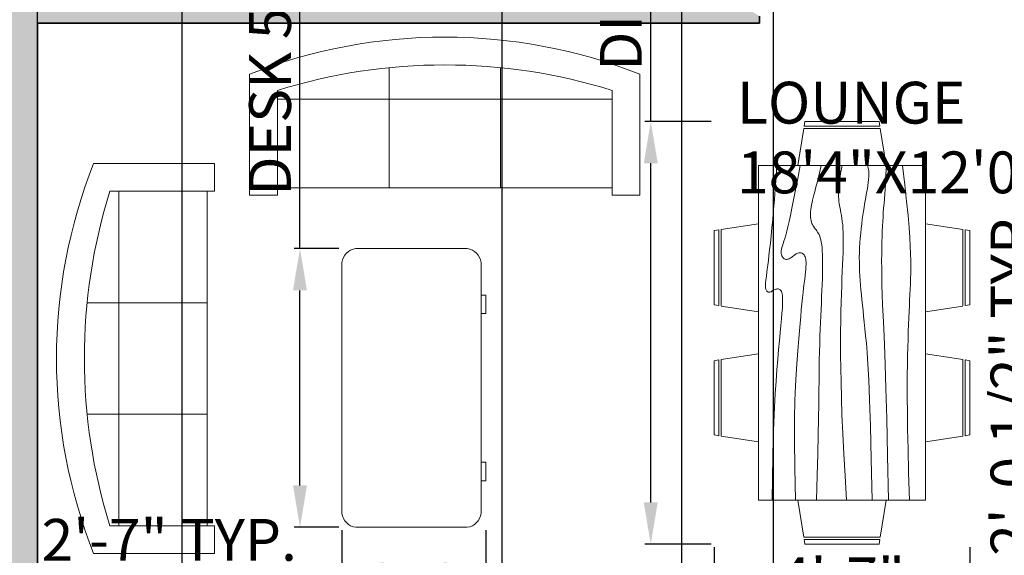
# Model space of a CAD drawing. Units: inches. Extents: x 32476 to 33108, y 58720 to 59630.
# Tile 4 of 6: x 32598 to 32810, y 59163 to 59278. Entities that reach past the tile are written whole.
import ezdxf

# ---------------------------------------------------------------- set-up
doc = ezdxf.new("R2010")
doc.units = ezdxf.units.IN
for name, color, linetype, lineweight in [('A-ANNO-DIMS', 6, 'Continuous', 18), ('A-AREA-IDEN', 32, 'Continuous', 18), ('A-FURN', 8, 'Continuous', 18), ('A-WALL', 7, 'Continuous', 35), ('A-WALL-PATT', 251, 'Continuous', 13)]:
    doc.layers.add(name, color=color, linetype=linetype, lineweight=lineweight)
doc.styles.get("Standard").update_dxf_attribs({"font": 'arial.ttf'})
doc.dimstyles.new('ISO-25', dxfattribs={"dimtxt": 9, "dimasz": 9, "dimexe": 1.25, "dimexo": 0.625, "dimtad": 1, "dimdec": 1, "dimrnd": 9, "dimlunit": 3, "dimtxsty": 'Standard', "dimcen": 2.5, "dimadec": 0, "dimazin": 0, "dimtfac": 1, "dimtdec": 1, "dimtmove": 0, "dimatfit": 3, "dimfxl": 1, "dimarcsym": 0})

# ---------------------------------------------------------------- blocks, each defined once
blk = doc.blocks.new('Sofa - Roundback 7 ft.')
for p, q in [((-12.00002, -32.4421), (-12.00003, -6.5971)), ((11.99997, -32.4421), (11.99998, -6.5971)), ((-36.000027, -34), (-36.000027, -11.4696)), ((35.99998, -34), (35.99998, -11.4696)), ((-35.999844, -13.3819), (35.9998, -13.3819)), ((-36.000027, -32.4421), (35.99998, -32.4421))]:
    blk.add_line(p, q)
for points in [[(-36.000027, -34), (-42.000027, -34), (-42.000027, -8)], [(41.99998, -8), (41.99998, -34), (35.99998, -34)]]:
    blk.add_lwpolyline(points)
for centre, radius, start, end in [((0, -114.25), 114.25, 68.43141, 111.5686), ((-0.00001, -127.1968), 121.1968, 72.72033, 107.2797)]:
    blk.add_arc(centre, radius, start, end)
blk = doc.blocks.new('Desk - 30 x 60 in.')
for p, q in [((-26.999995, 0), (26.999995, 0)), ((-29.999995, -27), (-29.999995, -3)), ((29.999995, -3), (29.999995, -27)), ((26.999995, -30), (-26.999995, -30)), ((-20.000005, -30), (-20.000005, -31)), ((-20.000005, -31), (-16.000005, -31)), ((-16.000005, -31), (-16.000005, -30)), ((15.999995, -31), (15.999995, -30)), ((19.999995, -31), (15.999995, -31)), ((19.999995, -30), (19.999995, -31))]:
    blk.add_line(p, q)
for centre, start, end in [((-26.499995, -3.5), 98.1301, 171.8699), ((26.499995, -3.5), 8.130102, 81.8699), ((-26.499995, -26.5), 188.1301, 261.8699), ((26.499995, -26.5), 278.1301, 351.8699)]:
    blk.add_arc(centre, 3.535534, start, end)
blk = doc.blocks.new('Dining Set - 36 x 72 in.')
for p, q in [((-22.2343, 26.00059), (-23.4847, 17.99762)), ((-22.2304, 26), (-5.7608, 26)), ((-22, 27.5), (-22.1562, 26.50042)), ((-5.8416, 26.5), (-22.1534, 26.5)), ((-22, 27.5), (-6, 27.5)), ((-5.8437, 26.49966), (-6, 27.5)), ((-4.5152, 17.99762), (-5.7655, 25.99926)), ((5.7657, 26.00059), (4.5153, 17.99762)), ((5.7696, 26), (22.2392, 26)), ((6, 27.5), (5.8438, 26.50042)), ((22.1584, 26.5), (5.8466, 26.5)), ((6, 27.5), (22, 27.5)), ((22.1563, 26.49966), (22, 27.5)), ((23.4848, 17.99762), (22.2345, 25.99926)), ((36, 18), (-36, 18)), ((-36, 18), (-36, -18)), ((36, -18), (36, 18)), ((-44.0006, 8.23428), (-35.9976, 9.48474)), ((44.0006, 8.23428), (35.9976, 9.48474)), ((-45.5, 8), (-44.5004, 8.15617)), ((-45.5, 8), (-45.5, -8)), ((-44.5, -8.15843), (-44.5, 8.15338)), ((-44, 8.23041), (-44, -8.23915)), ((44, 8.23041), (44, -8.23915)), ((44.5, -8.15843), (44.5, 8.15338)), ((45.5, 8), (44.5005, 8.15617)), ((45.5, 8), (45.5, -8)), ((-44.4997, -8.15631), (-45.5, -8)), ((-35.9976, -9.48476), (-43.9993, -8.2345)), ((35.9976, -9.48476), (43.9993, -8.2345)), ((44.4997, -8.15631), (45.5, -8)), ((-36, -18), (36, -18)), ((-22.2343, -26.0006), (-23.4847, -17.99762)), ((-4.5152, -17.99762), (-5.7655, -25.99928)), ((5.7657, -26.0006), (4.5153, -17.99762)), ((23.4848, -17.99762), (22.2345, -25.99928)), ((-22.2304, -26), (-5.7608, -26)), ((-22, -27.5), (-22.1562, -26.50044)), ((-5.8416, -26.5), (-22.1534, -26.5)), ((-22, -27.5), (-6, -27.5)), ((-5.8437, -26.49967), (-6, -27.5)), ((5.7696, -26), (22.2392, -26)), ((6, -27.5), (5.8438, -26.50044)), ((22.1584, -26.5), (5.8466, -26.5)), ((6, -27.5), (22, -27.5)), ((22.1563, -26.49967), (22, -27.5))]:
    blk.add_line(p, q)
for points in [[(-36, 15), (-31.1772, 14.97754), (-26.8079, 14.91406), (-22.8538, 14.81543), (-19.276, 14.6875), (-16.0362, 14.53613), (-13.0957, 14.36718), (-10.4159, 14.18652), (-7.9583, 14), (-5.6904, 13.81315), (-3.6035, 13.63021), (-1.6954, 13.45508), (0.0365, 13.29166), (1.5945, 13.14388), (2.9811, 13.01562), (4.1988, 12.9108), (5.25, 12.83333), (6.1393, 12.78613), (6.8802, 12.76823), (7.4883, 12.77767), (7.9792, 12.8125), (8.3685, 12.87077), (8.6719, 12.95052), (8.9049, 13.0498), (9.0833, 13.16666), (9.2205, 13.29899), (9.3216, 13.44401), (9.3895, 13.59879), (9.4271, 13.76041), (9.4373, 13.92594), (9.4232, 14.09245), (9.3875, 14.257), (9.3333, 14.41666), (9.2638, 14.56917), (9.1836, 14.71484), (9.0975, 14.85465), (9.0104, 14.98958), (8.9272, 15.1206), (8.8529, 15.2487), (8.7922, 15.37483), (8.75, 15.5), (8.7305, 15.62467), (8.7344, 15.74739), (8.7617, 15.86621), (8.8125, 15.97916), (8.8867, 16.08431), (8.9844, 16.17968), (9.1055, 16.26334), (9.25, 16.33333), (9.4189, 16.38802), (9.6172, 16.42708), (9.8506, 16.45052), (10.125, 16.45833), (10.4463, 16.45052), (10.8203, 16.42708), (11.2529, 16.38802), (11.75, 16.33333), (12.3184, 16.26318), (12.9694, 16.17838), (13.7151, 16.07991), (14.5677, 15.96875), (15.5395, 15.84586), (16.6426, 15.71224), (17.8893, 15.56884), (19.2917, 15.41666), (20.859, 15.25667), (22.5879, 15.08984), (24.4721, 14.91715), (26.5052, 14.73958), (28.6809, 14.5581), (30.9929, 14.3737), (33.4347, 14.18733), (36, 14)], [(-36, 10), (-28.9766, 10.14274), (-23.1725, 10.20442), (-18.4241, 10.19775), (-14.5677, 10.13541), (-11.4399, 10.03011), (-8.877, 9.89453), (-6.7154, 9.74137), (-4.7917, 9.58333), (-2.9698, 9.43082), (-1.2246, 9.28515), (0.4415, 9.14534), (2.026, 9.01041), (3.5266, 8.87939), (4.9408, 8.7513), (6.266, 8.62516), (7.5, 8.5), (8.6411, 8.37549), (9.6914, 8.2539), (10.6538, 8.13818), (11.5312, 8.03125), (12.3267, 7.93603), (13.043, 7.85547), (13.6831, 7.79248), (14.25, 7.75), (14.7471, 7.7303), (15.1797, 7.73307), (15.5537, 7.75732), (15.875, 7.80208), (16.1494, 7.86637), (16.3828, 7.94922), (16.5811, 8.04964), (16.75, 8.16666), (16.8944, 8.29915), (17.0143, 8.44531), (17.1089, 8.60319), (17.1771, 8.77083), (17.218, 8.94629), (17.2305, 9.1276), (17.2137, 9.31282), (17.1667, 9.5), (17.0895, 9.6875), (16.987, 9.875), (16.8649, 10.0625), (16.7292, 10.25), (16.5856, 10.4375), (16.4401, 10.625), (16.2985, 10.8125), (16.1667, 11), (16.05, 11.18733), (15.9518, 11.3737), (15.8752, 11.5581), (15.8229, 11.73958), (15.798, 11.91715), (15.8034, 12.08984), (15.842, 12.25667), (15.9167, 12.41666), (16.0295, 12.56836), (16.1784, 12.70833), (16.3605, 12.83268), (16.5729, 12.9375), (16.8127, 13.01888), (17.0768, 13.07291), (17.3625, 13.0957), (17.6667, 13.08333), (17.9894, 13.03312), (18.3418, 12.94726), (18.7382, 12.82918), (19.1927, 12.68229), (19.7195, 12.51001), (20.3327, 12.31575), (21.0465, 12.10294), (21.875, 11.875), (22.8357, 11.63354), (23.959, 11.37304), (25.2786, 11.08618), (26.8282, 10.76562), (28.6414, 10.40405), (30.752, 9.99414), (33.1936, 9.52856), (36, 9)], [(-36, 5.5), (-30.7157, 5.3348), (-26.069, 5.20963), (-21.9946, 5.11767), (-18.4271, 5.05208), (-15.3009, 5.00602), (-12.5508, 4.97265), (-10.1112, 4.94515), (-7.9167, 4.91666), (-5.909, 4.88167), (-4.0586, 4.83984), (-2.3429, 4.79215), (-0.7396, 4.73958), (0.7739, 4.6831), (2.22, 4.6237), (3.6213, 4.56233), (5, 4.5), (6.373, 4.43782), (7.7344, 4.3776), (9.0723, 4.32129), (10.375, 4.27083), (11.6309, 4.22819), (12.8281, 4.19531), (13.9551, 4.17415), (15, 4.16666), (15.954, 4.17448), (16.819, 4.19791), (17.6001, 4.23698), (18.3021, 4.29166), (18.9299, 4.36198), (19.4883, 4.44791), (19.9823, 4.54948), (20.4167, 4.66666), (20.7969, 4.79899), (21.1302, 4.94401), (21.4245, 5.09879), (21.6875, 5.26041), (21.9271, 5.42594), (22.1511, 5.59245), (22.3672, 5.757), (22.5834, 5.91666), (22.8065, 6.06868), (23.0404, 6.21093), (23.2879, 6.34147), (23.5521, 6.45833), (23.8358, 6.55957), (24.142, 6.64323), (24.4735, 6.70735), (24.8334, 6.75), (25.2235, 6.76969), (25.642, 6.76692), (26.0858, 6.74267), (26.5521, 6.69791), (27.0379, 6.63362), (27.5404, 6.55078), (28.0565, 6.45036), (28.5834, 6.33333), (29.1242, 6.19987), (29.7071, 6.04687), (30.3661, 5.87044), (31.1354, 5.66666), (32.0493, 5.43164), (33.142, 5.16146), (34.4475, 4.85221), (36, 4.5)], [(-36, -1), (-30.7915, -0.6591), (-26.0195, -0.38216), (-21.6519, -0.16284), (-17.6563, 0.00521), (-14.0005, 0.12833), (-10.6523, 0.21289), (-7.5796, 0.26522), (-4.75, 0.29166), (-2.134, 0.29793), (0.2878, 0.28711), (2.5317, 0.26163), (4.6146, 0.22396), (6.5529, 0.17651), (8.3633, 0.12174), (10.0623, 0.06209), (11.6667, 0), (13.1899, -0.06201), (14.6341, -0.1211), (15.9982, -0.17432), (17.2813, -0.21875), (18.4823, -0.25147), (19.6003, -0.26953), (20.6343, -0.27002), (21.5834, -0.25), (22.4481, -0.20768), (23.2357, -0.14584), (23.9549, -0.06836), (24.6146, 0.02083), (25.2235, 0.11784), (25.7904, 0.21875), (26.3241, 0.31966), (26.8334, 0.41666), (27.3265, 0.50618), (27.8099, 0.58593), (28.2894, 0.65397), (28.7709, 0.70833), (29.2601, 0.74707), (29.763, 0.76823), (30.2855, 0.76985), (30.8334, 0.75), (31.4088, 0.70784), (31.9994, 0.64713), (32.589, 0.57275), (33.1615, 0.48958), (33.7008, 0.4025), (34.1908, 0.3164), (34.6153, 0.23616), (34.9584, 0.16666), (35.2099, 0.11165), (35.3848, 0.07031), (35.504, 0.04069), (35.5886, 0.02083), (35.6594, 0.00879), (35.7377, 0.0026), (35.8442, 0.00032), (36, 0)], [(-36, -6.5), (-27.1843, -6.31267), (-20.084, -6.1263), (-14.469, -5.9419), (-10.1094, -5.76042), (-6.7752, -5.58285), (-4.2363, -5.41016), (-2.2629, -5.24333), (-0.625, -5.08334), (0.8708, -4.93099), (2.2715, -4.78646), (3.5872, -4.64974), (4.8281, -4.52084), (6.0046, -4.39974), (7.127, -4.28646), (8.2053, -4.18099), (9.25, -4.08334), (10.2705, -3.99382), (11.2734, -3.91407), (12.2647, -3.84603), (13.25, -3.79167), (14.2354, -3.75293), (15.2266, -3.73177), (16.2295, -3.73015), (17.25, -3.75), (18.2912, -3.79248), (19.3451, -3.85547), (20.4009, -3.93604), (21.4479, -4.03125), (22.4754, -4.13819), (23.4727, -4.25391), (24.4289, -4.37549), (25.3334, -4.5), (26.1785, -4.62492), (26.9694, -4.74935), (27.7145, -4.87281), (28.4219, -4.99479), (29.1, -5.11483), (29.7572, -5.23242), (30.4016, -5.34709), (31.0417, -5.45834), (31.6837, -5.56437), (32.3262, -5.65821), (32.9658, -5.73153), (33.599, -5.77604), (34.2224, -5.78345), (34.8327, -5.74545), (35.4264, -5.65373), (36, -5.5)], [(-36, -10), (-26.4022, -9.81299), (-18.4675, -9.62891), (-11.9839, -9.45069), (-6.7396, -9.28125), (-2.5226, -9.12354), (0.8789, -8.98047), (3.6769, -8.85498), (6.0833, -8.75), (8.2767, -8.66765), (10.3021, -8.60677), (12.1712, -8.56543), (13.8958, -8.54167), (15.4876, -8.53353), (16.9583, -8.53907), (18.3197, -8.55632), (19.5834, -8.58334), (20.7616, -8.61841), (21.8685, -8.66081), (22.9188, -8.71004), (23.9271, -8.76563), (24.9081, -8.82707), (25.8763, -8.89388), (26.8465, -8.96558), (27.8334, -9.04167), (28.8474, -9.12118), (29.8828, -9.20117), (30.93, -9.27824), (31.9792, -9.34896), (33.0205, -9.40991), (34.0443, -9.45768), (35.0407, -9.48885), (36, -9.5)], [(-36, -14.5), (-30.0881, -14.33513), (-25.0332, -14.21224), (-20.7312, -14.12647), (-17.0781, -14.07292), (-13.97, -14.04671), (-11.3027, -14.04297), (-8.9724, -14.05681), (-6.875, -14.08334), (-4.9224, -14.11833), (-3.0905, -14.16016), (-1.3709, -14.20785), (0.2448, -14.26042), (1.7647, -14.3169), (3.1973, -14.3763), (4.5507, -14.43767), (5.8333, -14.5), (7.0554, -14.5621), (8.235, -14.62175), (9.3922, -14.67652), (10.5469, -14.72396), (11.7192, -14.76164), (12.929, -14.78711), (14.1965, -14.79794), (15.5417, -14.79167), (16.9933, -14.76424), (18.6152, -14.70508), (20.4804, -14.60197), (22.6615, -14.44271), (25.2312, -14.21509), (28.2624, -13.9069), (31.8277, -13.50594), (36, -13)]]:
    blk.add_lwpolyline(points)
blk = doc.blocks.new('*D25')
at = {"layer": 'A-ANNO-DIMS', "color": 0, "lineweight": -2, "transparency": 16777216}
for p, q in [((32658.53, 59229.2), (32658.53, 59331.59)), ((32666.91, 59229.2), (32657.28, 59229.2)), ((32658.53, 59178.2), (32658.53, 59220.2)), ((32666.91, 59169.2), (32657.28, 59169.2))]:
    blk.add_line(p, q, dxfattribs=at)
at = {"layer": 'A-ANNO-DIMS', "color": 0, "transparency": 16777216}
for points in [[(32657.03, 59220.2), (32660.03, 59220.2), (32658.53, 59229.2)], [(32657.03, 59178.2), (32660.03, 59178.2), (32658.53, 59169.2)]]:
    blk.add_solid(points, dxfattribs=at)
at = {"layer": 'Defpoints', "color": 0, "transparency": 16777216}
for p in [(32658.53, 59229.2), (32667.53, 59229.2), (32667.53, 59169.2)]:
    blk.add_point(p, dxfattribs=at)
at = {"layer": 'A-ANNO-DIMS', "color": 0, "transparency": 16777216, "insert": (32653.25, 59284.89), "char_height": 9, "attachment_point": 5, "rotation": 90}
blk.add_mtext('DESK 5\'-0" TYP.', dxfattribs=at)
blk = doc.blocks.new('*D26')
at = {"layer": 'A-ANNO-DIMS', "color": 0, "lineweight": -2, "transparency": 16777216}
for p, q in [((32667.53, 59168.57), (32667.53, 59158.95)), ((32698.53, 59168.57), (32698.53, 59158.95)), ((32667.53, 59160.2), (32602.27, 59160.2)), ((32689.53, 59160.2), (32676.53, 59160.2))]:
    blk.add_line(p, q, dxfattribs=at)
at = {"layer": 'A-ANNO-DIMS', "color": 0, "transparency": 16777216}
for points in [[(32676.53, 59161.7), (32676.53, 59158.7), (32667.53, 59160.2)], [(32689.53, 59161.7), (32689.53, 59158.7), (32698.53, 59160.2)]]:
    blk.add_solid(points, dxfattribs=at)
at = {"layer": 'Defpoints', "color": 0, "transparency": 16777216}
for p in [(32667.53, 59169.2), (32698.53, 59169.2), (32667.53, 59160.2)]:
    blk.add_point(p, dxfattribs=at)
at = {"layer": 'A-ANNO-DIMS', "color": 0, "transparency": 16777216, "insert": (32630.4, 59165.34), "char_height": 9, "attachment_point": 5}
blk.add_mtext('2\'-7" TYP.', dxfattribs=at)
blk = doc.blocks.new('*D28')
at = {"layer": 'A-ANNO-DIMS', "color": 0, "lineweight": -2, "transparency": 16777216}
for p, q in [((32818.09, 59153.49), (32818.09, 59239.72)), ((32814.94, 59153.49), (32819.34, 59153.49)), ((32818.09, 59138.22), (32818.09, 59144.49)), ((32814.94, 59129.22), (32819.34, 59129.22))]:
    blk.add_line(p, q, dxfattribs=at)
at = {"layer": 'A-ANNO-DIMS', "color": 0, "transparency": 16777216}
for points in [[(32816.59, 59144.49), (32819.59, 59144.49), (32818.09, 59153.49)], [(32816.59, 59138.22), (32819.59, 59138.22), (32818.09, 59129.22)]]:
    blk.add_solid(points, dxfattribs=at)
at = {"layer": 'Defpoints', "color": 0, "transparency": 16777216}
for p in [(32814.31, 59153.49), (32818.09, 59153.49), (32814.31, 59129.22)]:
    blk.add_point(p, dxfattribs=at)
at = {"layer": 'A-ANNO-DIMS', "color": 0, "transparency": 16777216, "insert": (32812.81, 59201.11), "char_height": 9, "attachment_point": 5, "rotation": 90}
blk.add_mtext('2\'-0 1/2" TYP.', dxfattribs=at)
blk = doc.blocks.new('*D31')
at = {"layer": 'A-ANNO-DIMS', "color": 0, "lineweight": -2, "transparency": 16777216}
for p, q in [((32734.02, 59256.57), (32734.02, 59365.74)), ((32747.05, 59256.57), (32732.77, 59256.57)), ((32734.02, 59174.57), (32734.02, 59247.57)), ((32747.05, 59165.57), (32732.77, 59165.57))]:
    blk.add_line(p, q, dxfattribs=at)
at = {"layer": 'A-ANNO-DIMS', "color": 0, "transparency": 16777216}
for points in [[(32732.52, 59247.57), (32735.52, 59247.57), (32734.02, 59256.57)], [(32732.52, 59174.57), (32735.52, 59174.57), (32734.02, 59165.57)]]:
    blk.add_solid(points, dxfattribs=at)
at = {"layer": 'Defpoints', "color": 0, "transparency": 16777216}
for p in [(32734.02, 59256.57), (32747.67, 59256.57), (32747.67, 59165.57)]:
    blk.add_point(p, dxfattribs=at)
at = {"layer": 'A-ANNO-DIMS', "color": 0, "transparency": 16777216, "insert": (32728.75, 59315.65), "char_height": 9, "attachment_point": 5, "rotation": 90}
blk.add_mtext('DINING SET 7\'-7"', dxfattribs=at)
blk = doc.blocks.new('*D32')
at = {"layer": 'A-ANNO-DIMS', "color": 0, "lineweight": -2, "transparency": 16777216}
for p, q in [((32747.67, 59164.94), (32747.67, 59150.67)), ((32802.67, 59164.94), (32802.67, 59150.67)), ((32793.67, 59151.92), (32756.67, 59151.92))]:
    blk.add_line(p, q, dxfattribs=at)
at = {"layer": 'A-ANNO-DIMS', "color": 0, "transparency": 16777216}
for points in [[(32756.67, 59153.42), (32756.67, 59150.42), (32747.67, 59151.92)], [(32793.67, 59153.42), (32793.67, 59150.42), (32802.67, 59151.92)]]:
    blk.add_solid(points, dxfattribs=at)
at = {"layer": 'Defpoints', "color": 0, "transparency": 16777216}
for p in [(32747.67, 59165.57), (32802.67, 59165.57), (32747.67, 59151.92)]:
    blk.add_point(p, dxfattribs=at)
at = {"layer": 'A-ANNO-DIMS', "color": 0, "transparency": 16777216, "insert": (32775.17, 59157.04), "char_height": 9, "attachment_point": 5}
blk.add_mtext('4\'-7"', dxfattribs=at)
blk = doc.blocks.new('*D39')
at = {"layer": 'A-ANNO-DIMS', "color": 0, "lineweight": -2, "transparency": 16777216}
for p, q in [((32702.04, 59125.34), (32702.04, 59529.47)), ((32711.04, 59528.22), (32751.42, 59528.22)), ((32760.42, 59122.05), (32760.42, 59529.47))]:
    blk.add_line(p, q, dxfattribs=at)
at = {"layer": 'A-ANNO-DIMS', "color": 0, "transparency": 16777216}
for points in [[(32711.04, 59529.72), (32711.04, 59526.72), (32702.04, 59528.22)], [(32751.42, 59529.72), (32751.42, 59526.72), (32760.42, 59528.22)]]:
    blk.add_solid(points, dxfattribs=at)
at = {"layer": 'Defpoints', "color": 0, "transparency": 16777216}
for p in [(32760.42, 59528.22), (32702.04, 59124.72), (32760.42, 59121.43)]:
    blk.add_point(p, dxfattribs=at)
at = {"layer": 'A-ANNO-DIMS', "color": 0, "transparency": 16777216, "insert": (32731.23, 59533.5), "char_height": 9, "attachment_point": 5}
blk.add_mtext('4\'-10 1/2"', dxfattribs=at)
blk = doc.blocks.new('*D41')
at = {"layer": 'A-ANNO-DIMS', "color": 0, "lineweight": -2, "transparency": 16777216}
for p, q in [((32602.04, 59125.34), (32602.04, 59529.47)), ((32611.04, 59528.22), (32624.2, 59528.22)), ((32633.2, 59125.34), (32633.2, 59529.47))]:
    blk.add_line(p, q, dxfattribs=at)
at = {"layer": 'A-ANNO-DIMS', "color": 0, "transparency": 16777216}
for points in [[(32611.04, 59529.72), (32611.04, 59526.72), (32602.04, 59528.22)], [(32624.2, 59529.72), (32624.2, 59526.72), (32633.2, 59528.22)]]:
    blk.add_solid(points, dxfattribs=at)
at = {"layer": 'Defpoints', "color": 0, "transparency": 16777216}
for p in [(32633.2, 59528.22), (32602.04, 59124.72), (32633.2, 59124.72)]:
    blk.add_point(p, dxfattribs=at)
at = {"layer": 'A-ANNO-DIMS', "color": 0, "transparency": 16777216, "insert": (32617.62, 59533.36), "char_height": 9, "attachment_point": 5}
blk.add_mtext('2\'-7"', dxfattribs=at)
blk = doc.blocks.new('*D43')
at = {"layer": 'A-ANNO-DIMS', "color": 0, "lineweight": -2, "transparency": 16777216}
for p, q in [((32740.73, 58978.34), (32740.73, 59529.47)), ((32749.73, 59528.22), (32814.04, 59528.22)), ((32823.04, 58978.34), (32823.04, 59529.47))]:
    blk.add_line(p, q, dxfattribs=at)
at = {"layer": 'A-ANNO-DIMS', "color": 0, "transparency": 16777216}
for points in [[(32749.73, 59529.72), (32749.73, 59526.72), (32740.73, 59528.22)], [(32814.04, 59529.72), (32814.04, 59526.72), (32823.04, 59528.22)]]:
    blk.add_solid(points, dxfattribs=at)
at = {"layer": 'Defpoints', "color": 0, "transparency": 16777216}
for p in [(32823.04, 59528.22), (32740.73, 58977.72), (32823.04, 58977.72)]:
    blk.add_point(p, dxfattribs=at)
at = {"layer": 'A-ANNO-DIMS', "color": 0, "transparency": 16777216, "insert": (32781.88, 59533.5), "char_height": 9, "attachment_point": 5}
blk.add_mtext('6\'-10 1/2"', dxfattribs=at)

msp = doc.modelspace()

# ---------------------------------------------------------------- hatches: boundary and pattern name
at = {"layer": 'A-WALL-PATT'}
h = msp.add_hatch(color=256, dxfattribs=at)
h.dxf.hatch_style = 1
h.paths.add_polyline_path([(32602.04, 59418.72), (32606.39, 59418.72), (32606.39, 59423.22), (32602.04, 59423.22), (32602.04, 59477.22), (32698.04, 59477.22), (32698.04, 59469.73), (32702.54, 59469.73), (32702.54, 59481.72), (32867.54, 59481.72), (32867.54, 59427.72), (32860.2, 59427.72), (32860.2, 59418.72), (32867.54, 59418.72), (32935.14, 59418.72), (32935.14, 59423.22), (32872.04, 59423.22), (32872.04, 59477.22), (32968.04, 59477.22), (32968.04, 59423.22), (32962.36, 59423.22), (32962.36, 59418.72), (32968.04, 59418.72), (32968.04, 59286.72), (32867.54, 59286.72), (32832.04, 59286.72), (32828.7, 59289.44), (32818.99, 59279.82), (32823.04, 59277.72), (32823.04, 59269.52), (32832.04, 59269.52), (32832.04, 59277.72), (32867.54, 59277.72), (32968.04, 59277.72), (32968.04, 58880.22), (32925.88, 58880.22), (32925.88, 58871.22), (32968.04, 58871.22), (32968.04, 58799.22), (32823.04, 58799.22), (32823.04, 58790.22), (32977.04, 58790.22), (32977.04, 59486.22), (32867.54, 59486.22), (32702.54, 59486.22), (32593.04, 59486.22), (32593.04, 58803.66), (32602.04, 58803.66), (32602.04, 59001.72), (32624.39, 59001.72), (32624.39, 59010.72), (32602.04, 59010.72), (32602.04, 59124.72), (32648.65, 59124.72), (32648.65, 59133.72), (32602.04, 59133.72), (32602.04, 59277.72), (32757.41, 59277.72), (32757.41, 59279.22), (32742.07, 59288.84), (32739.6, 59286.72), (32702.54, 59286.72), (32602.04, 59286.72)])
h.paths.add_polyline_path([(32763.92, 59133.72), (32685.69, 59133.72), (32685.69, 59124.72), (32693.04, 59124.72), (32693.04, 59010.72), (32668.87, 59010.72), (32668.87, 59001.72), (32705.76, 59001.72), (32705.76, 59010.72), (32702.04, 59010.72), (32702.04, 59124.72), (32763.92, 59124.72)], flags=17)
h.paths.add_polyline_path([(32832.04, 59226.49), (32823.04, 59226.49), (32823.04, 59133.72), (32814.31, 59133.72), (32814.31, 59124.72), (32823.04, 59124.72), (32823.04, 59099.14), (32832.04, 59099.14), (32832.04, 59124.72), (32839.29, 59124.72), (32839.29, 59133.72), (32832.04, 59133.72)], flags=17)
h.paths.add_polyline_path([(32921.54, 59133.72), (32874.43, 59133.72), (32874.43, 59124.72), (32917.04, 59124.72), (32917.04, 59097.72), (32921.54, 59097.72), (32921.54, 59124.72)], flags=17)
h.paths.add_polyline_path([(32832.04, 59066.22), (32968.04, 59066.22), (32968.04, 59070.72), (32921.54, 59070.72), (32921.54, 59074.56), (32917.04, 59074.56), (32917.04, 59070.72), (32832.04, 59070.72), (32832.04, 59074.32), (32823.04, 59074.32), (32823.04, 59056.98), (32832.04, 59056.98)], flags=17)
h.paths.add_polyline_path([(32738.1, 59010.72), (32721.79, 59010.72), (32721.79, 59001.72), (32738.1, 59001.72)], flags=16)
h.paths.add_polyline_path([(32763.19, 59010.72), (32754.77, 59010.72), (32754.77, 59001.72), (32763.19, 59001.72)], flags=16)
h.paths.add_polyline_path([(32832.04, 59016.15), (32823.04, 59016.15), (32823.04, 59010.72), (32814.31, 59010.72), (32814.31, 59001.72), (32823.04, 59001.72), (32823.04, 58871.22), (32860.05, 58871.22), (32860.05, 58880.22), (32832.04, 58880.22)], flags=17)
h.paths.add_polyline_path([(32702.54, 59448.33), (32698.04, 59448.33), (32698.04, 59423.22), (32631.9, 59423.22), (32631.9, 59418.72), (32702.54, 59418.72), (32706.18, 59418.72), (32706.18, 59427.72), (32702.54, 59427.72)], flags=17)
h.paths.add_polyline_path([(32789.04, 59418.72), (32800.22, 59418.72), (32800.22, 59427.72), (32775.59, 59427.72), (32775.59, 59418.72), (32780.04, 59418.72), (32780.04, 59337.58), (32773.73, 59333.67), (32782.91, 59322.03), (32784.1, 59324.11), (32785.3, 59322.03), (32798.33, 59329.69), (32789.04, 59343.18)], flags=17)

# ---------------------------------------------------------------- linework, layer by layer
at = {"layer": 'A-WALL'}
for p, q in [((32757.41, 59277.72), (32757.41, 59279.22)), ((32757.41, 59277.72), (32602.04, 59277.72)), ((32602.04, 59277.72), (32602.04, 59133.72)), ((32702.54, 59277.72), (32757.41, 59277.72))]:
    msp.add_line(p, q, dxfattribs=at)

# ---------------------------------------------------------------- block references
at = {"layer": 'A-FURN'}
msp.add_blockref('Sofa - Roundback 7 ft.', (32689.7, 59274.73), dxfattribs=at)
at = {"layer": 'A-FURN', "rotation": 90}
for name, p in [('Dining Set - 36 x 72 in.', (32775.17, 59211.07)), ('Sofa - Roundback 7 ft.', (32606.13, 59205.54)), ('Desk - 30 x 60 in.', (32667.53, 59199.2))]:
    msp.add_blockref(name, p, dxfattribs=at)

# ---------------------------------------------------------------- texts
at = {"layer": 'A-AREA-IDEN', "insert": (32752.57, 59265.1), "char_height": 9, "attachment_point": 1}
msp.add_mtext_dynamic_manual_height_columns('LOUNGE\\P18\'4"X12\'0"', width=96.1811, gutter_width=12.5, heights=[0], dxfattribs=at)

# ---------------------------------------------------------------- dimensions: what is measured, and where the dimension line sits
at = {"layer": 'A-ANNO-DIMS'}
for base, p1, p2, picture, middle in [((32760.42, 59528.22), (32702.04, 59124.72), (32760.42, 59121.43), '*D39', (32731.23, 59533.5)), ((32823.04, 59528.22), (32740.73, 58977.72), (32823.04, 58977.72), '*D43', (32781.88, 59533.5)), ((32633.2, 59528.22), (32602.04, 59124.72), (32633.2, 59124.72), '*D41', (32617.62, 59533.36))]:
    dim = msp.add_linear_dim(base=base, p1=p1, p2=p2, dimstyle='ISO-25', override={"dimdec": 1, "dimlfac": 1, "dimrnd": 0, "dimzin": 1, "dimdsep": 46, "dimlunit": 4, "dimfrac": 2}, dxfattribs=at)
    dim.commit()
    dim.dimension.update_dxf_attribs({"geometry": picture, "text_midpoint": middle})
for base, p1, p2, angle, text, picture, middle in [((32734.02, 59256.57), (32747.67, 59165.57), (32747.67, 59256.57), 90, 'DINING SET <>', '*D31', (32728.75, 59315.65)), ((32658.53, 59229.2), (32667.53, 59169.2), (32667.53, 59229.2), 90, 'DESK <> TYP.', '*D25', (32653.25, 59284.89)), ((32818.09, 59153.49), (32814.31, 59129.22), (32814.31, 59153.49), 90, '<> TYP.', '*D28', (32812.81, 59201.11)), ((32667.53, 59160.2), (32698.53, 59169.2), (32667.53, 59169.2), 180, '<> TYP.', '*D26', (32630.4, 59165.34))]:
    dim = msp.add_linear_dim(base=base, p1=p1, p2=p2, angle=angle, text=text, dimstyle='ISO-25', override={"dimdec": 1, "dimlfac": 1, "dimrnd": 0, "dimzin": 1, "dimdsep": 46, "dimlunit": 4, "dimfrac": 2}, dxfattribs=at)
    dim.commit()
    dim.dimension.update_dxf_attribs({"geometry": picture, "text_midpoint": middle})
dim = msp.add_linear_dim(base=(32747.67, 59151.92), p1=(32802.67, 59165.57), p2=(32747.67, 59165.57), angle=180, dimstyle='ISO-25', override={"dimdec": 1, "dimlfac": 1, "dimrnd": 0, "dimzin": 1, "dimdsep": 46, "dimlunit": 4, "dimfrac": 2}, dxfattribs=at)
dim.commit()
dim.dimension.update_dxf_attribs({"geometry": '*D32', "text_midpoint": (32775.17, 59157.04)})

doc.saveas('drawing.dxf')
